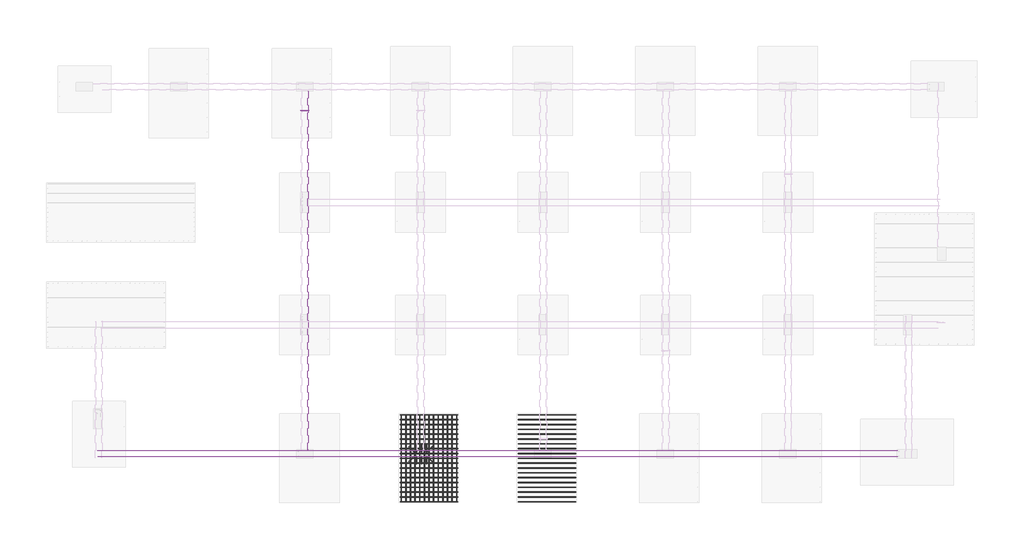
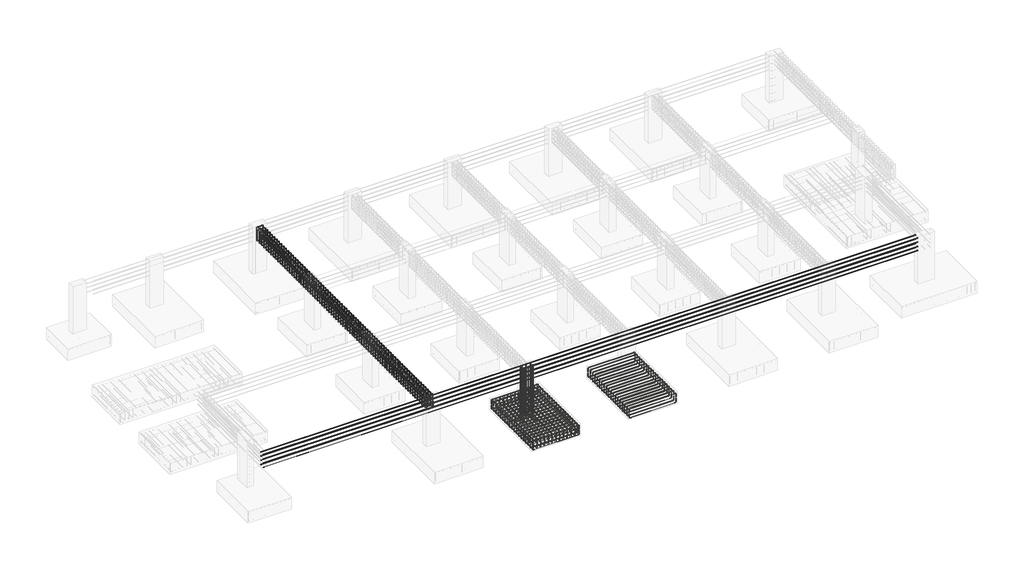
# One storey, part 4 of 16: 16 reinforcing bars.
"""IFC4 building model written with IfcOpenShell, lengths in millimetres."""

from ifc_helpers import new_model, si_unit, point, frame, origin, place, context, project, spatial, polyline, circle_curve, trimmed, segment, composite_curve, source, transform, mapped, element, save
from ifc_brep_helpers import swept_disk

model = new_model("IFC4")

# Units and contexts
model_context = context("Model", 3, world=origin())
ifc_project = project(units=[si_unit("LENGTHUNIT", "METRE", prefix="MILLI")], contexts=[model_context])

# Site, building, storey
site = spatial("IfcSite", under=ifc_project)
building = spatial("IfcBuilding", under=site)
storey = spatial("IfcBuildingStorey", under=building, Elevation=-1828.8)

# Reinforcing bars
placement = place(None, origin())
reinforcing_bar_shape = source(origin(), model_context, "Body", "SolidModel", [
    swept_disk(composite_curve([segment(polyline([(-744.0266166, -5094.4085501, -2088.8), (-744.0266166, -5094.4085501, -2212.8)]), True, "CONTINUOUS"), segment(trimmed(circle_curve(frame((-774.0266166, -5094.4085501, -2212.8), z_axis=(0.0, 1.0, 0.0), x_axis=(30.0, 0.0, 0.0)), 30.0), [point((-744.0266166, -5094.4085501, -2212.8))], [point((-774.0266166, -5094.4085501, -2242.8))], True, "CARTESIAN"), True, "CONTINUOUS"), segment(polyline([(-774.0266166, -5094.4085501, -2242.8), (-2442.0266166, -5094.4085501, -2242.8)]), True, "CONTINUOUS"), segment(trimmed(circle_curve(frame((-2442.0266166, -5094.4085501, -2212.8), z_axis=(0.0, 1.0, 0.0), x_axis=(0.0, 0.0, -30.0)), 30.0), [point((-2442.0266166, -5094.4085501, -2242.8))], [point((-2472.0266166, -5094.4085501, -2212.8))], True, "CARTESIAN"), True, "CONTINUOUS"), segment(polyline([(-2472.0266166, -5094.4085501, -2212.8), (-2472.0266166, -5094.4085501, -2088.8)]), True, "CONTINUOUS")], self_intersect=False), 6.0),
])
element("IfcReinforcingBar", 1, at=placement, inside=storey, context=model_context, shape_type="MappedRepresentation", body=[
    mapped(reinforcing_bar_shape, transform((0.0, 0.0, 0.0), x_axis=(1.0, 0.0, 0.0), y_axis=(0.0, 1.0, 0.0), z_axis=(0.0, 0.0, 1.0))),
    mapped(reinforcing_bar_shape, transform((0.0, -146.0, 0.0), x_axis=(1.0, 0.0, 0.0), y_axis=(0.0, 1.0, 0.0), z_axis=(0.0, 0.0, 1.0))),
    mapped(reinforcing_bar_shape, transform((0.0, -292.0, 0.0), x_axis=(1.0, 0.0, 0.0), y_axis=(0.0, 1.0, 0.0), z_axis=(0.0, 0.0, 1.0))),
    mapped(reinforcing_bar_shape, transform((0.0, -438.0, 0.0), x_axis=(1.0, 0.0, 0.0), y_axis=(0.0, 1.0, 0.0), z_axis=(0.0, 0.0, 1.0))),
    mapped(reinforcing_bar_shape, transform((0.0, -584.0, 0.0), x_axis=(1.0, 0.0, 0.0), y_axis=(0.0, 1.0, 0.0), z_axis=(0.0, 0.0, 1.0))),
    mapped(reinforcing_bar_shape, transform((0.0, -730.0, 0.0), x_axis=(1.0, 0.0, 0.0), y_axis=(0.0, 1.0, 0.0), z_axis=(0.0, 0.0, 1.0))),
    mapped(reinforcing_bar_shape, transform((0.0, -876.0, 0.0), x_axis=(1.0, 0.0, 0.0), y_axis=(0.0, 1.0, 0.0), z_axis=(0.0, 0.0, 1.0))),
    mapped(reinforcing_bar_shape, transform((0.0, -1022.0, 0.0), x_axis=(1.0, 0.0, 0.0), y_axis=(0.0, 1.0, 0.0), z_axis=(0.0, 0.0, 1.0))),
    mapped(reinforcing_bar_shape, transform((0.0, -1168.0, 0.0), x_axis=(1.0, 0.0, 0.0), y_axis=(0.0, 1.0, 0.0), z_axis=(0.0, 0.0, 1.0))),
    mapped(reinforcing_bar_shape, transform((0.0, -1314.0, 0.0), x_axis=(1.0, 0.0, 0.0), y_axis=(0.0, 1.0, 0.0), z_axis=(0.0, 0.0, 1.0))),
    mapped(reinforcing_bar_shape, transform((0.0, -1460.0, 0.0), x_axis=(1.0, 0.0, 0.0), y_axis=(0.0, 1.0, 0.0), z_axis=(0.0, 0.0, 1.0))),
    mapped(reinforcing_bar_shape, transform((0.0, -1606.0, 0.0), x_axis=(1.0, 0.0, 0.0), y_axis=(0.0, 1.0, 0.0), z_axis=(0.0, 0.0, 1.0))),
    mapped(reinforcing_bar_shape, transform((0.0, -1752.0, 0.0), x_axis=(1.0, 0.0, 0.0), y_axis=(0.0, 1.0, 0.0), z_axis=(0.0, 0.0, 1.0))),
    mapped(reinforcing_bar_shape, transform((0.0, -1898.0, 0.0), x_axis=(1.0, 0.0, 0.0), y_axis=(0.0, 1.0, 0.0), z_axis=(0.0, 0.0, 1.0))),
    mapped(reinforcing_bar_shape, transform((0.0, -2044.0, 0.0), x_axis=(1.0, 0.0, 0.0), y_axis=(0.0, 1.0, 0.0), z_axis=(0.0, 0.0, 1.0))),
    mapped(reinforcing_bar_shape, transform((0.0, -2190.0, 0.0), x_axis=(1.0, 0.0, 0.0), y_axis=(0.0, 1.0, 0.0), z_axis=(0.0, 0.0, 1.0))),
    mapped(reinforcing_bar_shape, transform((0.0, -2336.0, 0.0), x_axis=(1.0, 0.0, 0.0), y_axis=(0.0, 1.0, 0.0), z_axis=(0.0, 0.0, 1.0))),
    mapped(reinforcing_bar_shape, transform((0.0, -2482.0, 0.0), x_axis=(1.0, 0.0, 0.0), y_axis=(0.0, 1.0, 0.0), z_axis=(0.0, 0.0, 1.0))),
    mapped(reinforcing_bar_shape, transform((0.0, -2628.0, 0.0), x_axis=(1.0, 0.0, 0.0), y_axis=(0.0, 1.0, 0.0), z_axis=(0.0, 0.0, 1.0))),
])
reinforcing_bar_2_shape = source(origin(), model_context, "Body", "SolidModel", [
    swept_disk(composite_curve([segment(polyline([(-2472.0266166, -5094.4085501, -2024.671783), (-2472.0266166, -5094.4085501, -1900.671783)]), True, "CONTINUOUS"), segment(trimmed(circle_curve(frame((-2442.0266166, -5094.4085501, -1900.671783), z_axis=(0.0, 1.0, 0.0), x_axis=(-30.0, 0.0, 0.0)), 30.0), [point((-2472.0266166, -5094.4085501, -1900.671783))], [point((-2442.0266166, -5094.4085501, -1870.671783))], True, "CARTESIAN"), True, "CONTINUOUS"), segment(polyline([(-2442.0266166, -5094.4085501, -1870.671783), (-774.0266166, -5094.4085501, -1870.671783)]), True, "CONTINUOUS"), segment(trimmed(circle_curve(frame((-774.0266166, -5094.4085501, -1900.671783), z_axis=(0.0, 1.0, 0.0), x_axis=(0.0, 0.0, 30.0)), 30.0), [point((-774.0266166, -5094.4085501, -1870.671783))], [point((-744.0266166, -5094.4085501, -1900.671783))], True, "CARTESIAN"), True, "CONTINUOUS"), segment(polyline([(-744.0266166, -5094.4085501, -1900.671783), (-744.0266166, -5094.4085501, -2024.671783)]), True, "CONTINUOUS")], self_intersect=False), 6.0),
])
element("IfcReinforcingBar", 2, at=placement, inside=storey, context=model_context, shape_type="MappedRepresentation", body=[
    mapped(reinforcing_bar_2_shape, transform((0.0, 0.0, 0.0), x_axis=(1.0, 0.0, 0.0), y_axis=(0.0, 1.0, 0.0), z_axis=(0.0, 0.0, 1.0))),
    mapped(reinforcing_bar_2_shape, transform((0.0, -146.0, 0.0), x_axis=(1.0, 0.0, 0.0), y_axis=(0.0, 1.0, 0.0), z_axis=(0.0, 0.0, 1.0))),
    mapped(reinforcing_bar_2_shape, transform((0.0, -292.0, 0.0), x_axis=(1.0, 0.0, 0.0), y_axis=(0.0, 1.0, 0.0), z_axis=(0.0, 0.0, 1.0))),
    mapped(reinforcing_bar_2_shape, transform((0.0, -438.0, 0.0), x_axis=(1.0, 0.0, 0.0), y_axis=(0.0, 1.0, 0.0), z_axis=(0.0, 0.0, 1.0))),
    mapped(reinforcing_bar_2_shape, transform((0.0, -584.0, 0.0), x_axis=(1.0, 0.0, 0.0), y_axis=(0.0, 1.0, 0.0), z_axis=(0.0, 0.0, 1.0))),
    mapped(reinforcing_bar_2_shape, transform((0.0, -730.0, 0.0), x_axis=(1.0, 0.0, 0.0), y_axis=(0.0, 1.0, 0.0), z_axis=(0.0, 0.0, 1.0))),
    mapped(reinforcing_bar_2_shape, transform((0.0, -876.0, 0.0), x_axis=(1.0, 0.0, 0.0), y_axis=(0.0, 1.0, 0.0), z_axis=(0.0, 0.0, 1.0))),
    mapped(reinforcing_bar_2_shape, transform((0.0, -1022.0, 0.0), x_axis=(1.0, 0.0, 0.0), y_axis=(0.0, 1.0, 0.0), z_axis=(0.0, 0.0, 1.0))),
    mapped(reinforcing_bar_2_shape, transform((0.0, -1168.0, 0.0), x_axis=(1.0, 0.0, 0.0), y_axis=(0.0, 1.0, 0.0), z_axis=(0.0, 0.0, 1.0))),
    mapped(reinforcing_bar_2_shape, transform((0.0, -1314.0, 0.0), x_axis=(1.0, 0.0, 0.0), y_axis=(0.0, 1.0, 0.0), z_axis=(0.0, 0.0, 1.0))),
    mapped(reinforcing_bar_2_shape, transform((0.0, -1460.0, 0.0), x_axis=(1.0, 0.0, 0.0), y_axis=(0.0, 1.0, 0.0), z_axis=(0.0, 0.0, 1.0))),
    mapped(reinforcing_bar_2_shape, transform((0.0, -1606.0, 0.0), x_axis=(1.0, 0.0, 0.0), y_axis=(0.0, 1.0, 0.0), z_axis=(0.0, 0.0, 1.0))),
    mapped(reinforcing_bar_2_shape, transform((0.0, -1752.0, 0.0), x_axis=(1.0, 0.0, 0.0), y_axis=(0.0, 1.0, 0.0), z_axis=(0.0, 0.0, 1.0))),
    mapped(reinforcing_bar_2_shape, transform((0.0, -1898.0, 0.0), x_axis=(1.0, 0.0, 0.0), y_axis=(0.0, 1.0, 0.0), z_axis=(0.0, 0.0, 1.0))),
    mapped(reinforcing_bar_2_shape, transform((0.0, -2044.0, 0.0), x_axis=(1.0, 0.0, 0.0), y_axis=(0.0, 1.0, 0.0), z_axis=(0.0, 0.0, 1.0))),
    mapped(reinforcing_bar_2_shape, transform((0.0, -2190.0, 0.0), x_axis=(1.0, 0.0, 0.0), y_axis=(0.0, 1.0, 0.0), z_axis=(0.0, 0.0, 1.0))),
    mapped(reinforcing_bar_2_shape, transform((0.0, -2336.0, 0.0), x_axis=(1.0, 0.0, 0.0), y_axis=(0.0, 1.0, 0.0), z_axis=(0.0, 0.0, 1.0))),
    mapped(reinforcing_bar_2_shape, transform((0.0, -2482.0, 0.0), x_axis=(1.0, 0.0, 0.0), y_axis=(0.0, 1.0, 0.0), z_axis=(0.0, 0.0, 1.0))),
    mapped(reinforcing_bar_2_shape, transform((0.0, -2628.0, 0.0), x_axis=(1.0, 0.0, 0.0), y_axis=(0.0, 1.0, 0.0), z_axis=(0.0, 0.0, 1.0))),
])
reinforcing_bar_3_shape = source(origin(), model_context, "Body", "SolidModel", [
    swept_disk(composite_curve([segment(polyline([(-4314.2725801, -5094.4085501, -2088.8), (-4314.2725801, -5094.4085501, -2212.8)]), True, "CONTINUOUS"), segment(trimmed(circle_curve(frame((-4344.2725801, -5094.4085501, -2212.8), z_axis=(0.0, 1.0, 0.0), x_axis=(30.0, 0.0, 0.0)), 30.0), [point((-4314.2725801, -5094.4085501, -2212.8))], [point((-4344.2725801, -5094.4085501, -2242.8))], True, "CARTESIAN"), True, "CONTINUOUS"), segment(polyline([(-4344.2725801, -5094.4085501, -2242.8), (-6012.2725801, -5094.4085501, -2242.8)]), True, "CONTINUOUS"), segment(trimmed(circle_curve(frame((-6012.2725801, -5094.4085501, -2212.8), z_axis=(0.0, 1.0, 0.0), x_axis=(0.0, 0.0, -30.0)), 30.0), [point((-6012.2725801, -5094.4085501, -2242.8))], [point((-6042.2725801, -5094.4085501, -2212.8))], True, "CARTESIAN"), True, "CONTINUOUS"), segment(polyline([(-6042.2725801, -5094.4085501, -2212.8), (-6042.2725801, -5094.4085501, -2088.8)]), True, "CONTINUOUS")], self_intersect=False), 6.0),
])
element("IfcReinforcingBar", 3, at=placement, inside=storey, context=model_context, shape_type="MappedRepresentation", body=[
    mapped(reinforcing_bar_3_shape, transform((0.0, 0.0, 0.0), x_axis=(1.0, 0.0, 0.0), y_axis=(0.0, 1.0, 0.0), z_axis=(0.0, 0.0, 1.0))),
    mapped(reinforcing_bar_3_shape, transform((0.0, -146.0, 0.0), x_axis=(1.0, 0.0, 0.0), y_axis=(0.0, 1.0, 0.0), z_axis=(0.0, 0.0, 1.0))),
    mapped(reinforcing_bar_3_shape, transform((0.0, -292.0, 0.0), x_axis=(1.0, 0.0, 0.0), y_axis=(0.0, 1.0, 0.0), z_axis=(0.0, 0.0, 1.0))),
    mapped(reinforcing_bar_3_shape, transform((0.0, -438.0, 0.0), x_axis=(1.0, 0.0, 0.0), y_axis=(0.0, 1.0, 0.0), z_axis=(0.0, 0.0, 1.0))),
    mapped(reinforcing_bar_3_shape, transform((0.0, -584.0, 0.0), x_axis=(1.0, 0.0, 0.0), y_axis=(0.0, 1.0, 0.0), z_axis=(0.0, 0.0, 1.0))),
    mapped(reinforcing_bar_3_shape, transform((0.0, -730.0, 0.0), x_axis=(1.0, 0.0, 0.0), y_axis=(0.0, 1.0, 0.0), z_axis=(0.0, 0.0, 1.0))),
    mapped(reinforcing_bar_3_shape, transform((0.0, -876.0, 0.0), x_axis=(1.0, 0.0, 0.0), y_axis=(0.0, 1.0, 0.0), z_axis=(0.0, 0.0, 1.0))),
    mapped(reinforcing_bar_3_shape, transform((0.0, -1022.0, 0.0), x_axis=(1.0, 0.0, 0.0), y_axis=(0.0, 1.0, 0.0), z_axis=(0.0, 0.0, 1.0))),
    mapped(reinforcing_bar_3_shape, transform((0.0, -1168.0, 0.0), x_axis=(1.0, 0.0, 0.0), y_axis=(0.0, 1.0, 0.0), z_axis=(0.0, 0.0, 1.0))),
    mapped(reinforcing_bar_3_shape, transform((0.0, -1314.0, 0.0), x_axis=(1.0, 0.0, 0.0), y_axis=(0.0, 1.0, 0.0), z_axis=(0.0, 0.0, 1.0))),
    mapped(reinforcing_bar_3_shape, transform((0.0, -1460.0, 0.0), x_axis=(1.0, 0.0, 0.0), y_axis=(0.0, 1.0, 0.0), z_axis=(0.0, 0.0, 1.0))),
    mapped(reinforcing_bar_3_shape, transform((0.0, -1606.0, 0.0), x_axis=(1.0, 0.0, 0.0), y_axis=(0.0, 1.0, 0.0), z_axis=(0.0, 0.0, 1.0))),
    mapped(reinforcing_bar_3_shape, transform((0.0, -1752.0, 0.0), x_axis=(1.0, 0.0, 0.0), y_axis=(0.0, 1.0, 0.0), z_axis=(0.0, 0.0, 1.0))),
    mapped(reinforcing_bar_3_shape, transform((0.0, -1898.0, 0.0), x_axis=(1.0, 0.0, 0.0), y_axis=(0.0, 1.0, 0.0), z_axis=(0.0, 0.0, 1.0))),
    mapped(reinforcing_bar_3_shape, transform((0.0, -2044.0, 0.0), x_axis=(1.0, 0.0, 0.0), y_axis=(0.0, 1.0, 0.0), z_axis=(0.0, 0.0, 1.0))),
    mapped(reinforcing_bar_3_shape, transform((0.0, -2190.0, 0.0), x_axis=(1.0, 0.0, 0.0), y_axis=(0.0, 1.0, 0.0), z_axis=(0.0, 0.0, 1.0))),
    mapped(reinforcing_bar_3_shape, transform((0.0, -2336.0, 0.0), x_axis=(1.0, 0.0, 0.0), y_axis=(0.0, 1.0, 0.0), z_axis=(0.0, 0.0, 1.0))),
    mapped(reinforcing_bar_3_shape, transform((0.0, -2482.0, 0.0), x_axis=(1.0, 0.0, 0.0), y_axis=(0.0, 1.0, 0.0), z_axis=(0.0, 0.0, 1.0))),
    mapped(reinforcing_bar_3_shape, transform((0.0, -2628.0, 0.0), x_axis=(1.0, 0.0, 0.0), y_axis=(0.0, 1.0, 0.0), z_axis=(0.0, 0.0, 1.0))),
])
reinforcing_bar_4_shape = source(origin(), model_context, "Body", "SolidModel", [
    swept_disk(composite_curve([segment(polyline([(-6042.2725801, -5094.4085501, -2024.671783), (-6042.2725801, -5094.4085501, -1900.671783)]), True, "CONTINUOUS"), segment(trimmed(circle_curve(frame((-6012.2725801, -5094.4085501, -1900.671783), z_axis=(0.0, 1.0, 0.0), x_axis=(-30.0, 0.0, 0.0)), 30.0), [point((-6042.2725801, -5094.4085501, -1900.671783))], [point((-6012.2725801, -5094.4085501, -1870.671783))], True, "CARTESIAN"), True, "CONTINUOUS"), segment(polyline([(-6012.2725801, -5094.4085501, -1870.671783), (-4344.2725801, -5094.4085501, -1870.671783)]), True, "CONTINUOUS"), segment(trimmed(circle_curve(frame((-4344.2725801, -5094.4085501, -1900.671783), z_axis=(0.0, 1.0, 0.0), x_axis=(0.0, 0.0, 30.0)), 30.0), [point((-4344.2725801, -5094.4085501, -1870.671783))], [point((-4314.2725801, -5094.4085501, -1900.671783))], True, "CARTESIAN"), True, "CONTINUOUS"), segment(polyline([(-4314.2725801, -5094.4085501, -1900.671783), (-4314.2725801, -5094.4085501, -2024.671783)]), True, "CONTINUOUS")], self_intersect=False), 6.0),
])
element("IfcReinforcingBar", 4, at=placement, inside=storey, context=model_context, shape_type="MappedRepresentation", body=[
    mapped(reinforcing_bar_4_shape, transform((0.0, 0.0, 0.0), x_axis=(1.0, 0.0, 0.0), y_axis=(0.0, 1.0, 0.0), z_axis=(0.0, 0.0, 1.0))),
    mapped(reinforcing_bar_4_shape, transform((0.0, -146.0, 0.0), x_axis=(1.0, 0.0, 0.0), y_axis=(0.0, 1.0, 0.0), z_axis=(0.0, 0.0, 1.0))),
    mapped(reinforcing_bar_4_shape, transform((0.0, -292.0, 0.0), x_axis=(1.0, 0.0, 0.0), y_axis=(0.0, 1.0, 0.0), z_axis=(0.0, 0.0, 1.0))),
    mapped(reinforcing_bar_4_shape, transform((0.0, -438.0, 0.0), x_axis=(1.0, 0.0, 0.0), y_axis=(0.0, 1.0, 0.0), z_axis=(0.0, 0.0, 1.0))),
    mapped(reinforcing_bar_4_shape, transform((0.0, -584.0, 0.0), x_axis=(1.0, 0.0, 0.0), y_axis=(0.0, 1.0, 0.0), z_axis=(0.0, 0.0, 1.0))),
    mapped(reinforcing_bar_4_shape, transform((0.0, -730.0, 0.0), x_axis=(1.0, 0.0, 0.0), y_axis=(0.0, 1.0, 0.0), z_axis=(0.0, 0.0, 1.0))),
    mapped(reinforcing_bar_4_shape, transform((0.0, -876.0, 0.0), x_axis=(1.0, 0.0, 0.0), y_axis=(0.0, 1.0, 0.0), z_axis=(0.0, 0.0, 1.0))),
    mapped(reinforcing_bar_4_shape, transform((0.0, -1022.0, 0.0), x_axis=(1.0, 0.0, 0.0), y_axis=(0.0, 1.0, 0.0), z_axis=(0.0, 0.0, 1.0))),
    mapped(reinforcing_bar_4_shape, transform((0.0, -1168.0, 0.0), x_axis=(1.0, 0.0, 0.0), y_axis=(0.0, 1.0, 0.0), z_axis=(0.0, 0.0, 1.0))),
    mapped(reinforcing_bar_4_shape, transform((0.0, -1314.0, 0.0), x_axis=(1.0, 0.0, 0.0), y_axis=(0.0, 1.0, 0.0), z_axis=(0.0, 0.0, 1.0))),
    mapped(reinforcing_bar_4_shape, transform((0.0, -1460.0, 0.0), x_axis=(1.0, 0.0, 0.0), y_axis=(0.0, 1.0, 0.0), z_axis=(0.0, 0.0, 1.0))),
    mapped(reinforcing_bar_4_shape, transform((0.0, -1606.0, 0.0), x_axis=(1.0, 0.0, 0.0), y_axis=(0.0, 1.0, 0.0), z_axis=(0.0, 0.0, 1.0))),
    mapped(reinforcing_bar_4_shape, transform((0.0, -1752.0, 0.0), x_axis=(1.0, 0.0, 0.0), y_axis=(0.0, 1.0, 0.0), z_axis=(0.0, 0.0, 1.0))),
    mapped(reinforcing_bar_4_shape, transform((0.0, -1898.0, 0.0), x_axis=(1.0, 0.0, 0.0), y_axis=(0.0, 1.0, 0.0), z_axis=(0.0, 0.0, 1.0))),
    mapped(reinforcing_bar_4_shape, transform((0.0, -2044.0, 0.0), x_axis=(1.0, 0.0, 0.0), y_axis=(0.0, 1.0, 0.0), z_axis=(0.0, 0.0, 1.0))),
    mapped(reinforcing_bar_4_shape, transform((0.0, -2190.0, 0.0), x_axis=(1.0, 0.0, 0.0), y_axis=(0.0, 1.0, 0.0), z_axis=(0.0, 0.0, 1.0))),
    mapped(reinforcing_bar_4_shape, transform((0.0, -2336.0, 0.0), x_axis=(1.0, 0.0, 0.0), y_axis=(0.0, 1.0, 0.0), z_axis=(0.0, 0.0, 1.0))),
    mapped(reinforcing_bar_4_shape, transform((0.0, -2482.0, 0.0), x_axis=(1.0, 0.0, 0.0), y_axis=(0.0, 1.0, 0.0), z_axis=(0.0, 0.0, 1.0))),
    mapped(reinforcing_bar_4_shape, transform((0.0, -2628.0, 0.0), x_axis=(1.0, 0.0, 0.0), y_axis=(0.0, 1.0, 0.0), z_axis=(0.0, 0.0, 1.0))),
])
reinforcing_bar_5_shape = source(origin(), model_context, "Body", "SolidModel", [
    swept_disk(composite_curve([segment(polyline([(-6015.8984804, -5094.4085501, -2074.8303715), (-6015.8984804, -5094.4085501, -2198.8303715)]), True, "CONTINUOUS"), segment(trimmed(circle_curve(frame((-6015.8984804, -5124.4085501, -2198.8303715), z_axis=(-1.0, 0.0, 0.0), x_axis=(0.0, 30.0, 0.0)), 30.0), [point((-6015.8984804, -5094.4085501, -2198.8303715))], [point((-6015.8984804, -5124.4085501, -2228.8303715))], True, "CARTESIAN"), True, "CONTINUOUS"), segment(polyline([(-6015.8984804, -5124.4085501, -2228.8303715), (-6015.8984804, -7692.4085501, -2228.8303715)]), True, "CONTINUOUS"), segment(trimmed(circle_curve(frame((-6015.8984804, -7692.4085501, -2198.8303715), z_axis=(-1.0, 0.0, 0.0), x_axis=(0.0, 0.0, -30.0)), 30.0), [point((-6015.8984804, -7692.4085501, -2228.8303715))], [point((-6015.8984804, -7722.4085501, -2198.8303715))], True, "CARTESIAN"), True, "CONTINUOUS"), segment(polyline([(-6015.8984804, -7722.4085501, -2198.8303715), (-6015.8984804, -7722.4085501, -2074.8303715)]), True, "CONTINUOUS")], self_intersect=False), 6.0),
])
element("IfcReinforcingBar", 5, at=placement, inside=storey, context=model_context, shape_type="MappedRepresentation", body=[
    mapped(reinforcing_bar_5_shape, transform((0.0, 0.0, 0.0), x_axis=(1.0, 0.0, 0.0), y_axis=(0.0, 1.0, 0.0), z_axis=(0.0, 0.0, 1.0))),
    mapped(reinforcing_bar_5_shape, transform((139.7704391, 0.0, 0.0), x_axis=(1.0, 0.0, 0.0), y_axis=(0.0, 1.0, 0.0), z_axis=(0.0, 0.0, 1.0))),
    mapped(reinforcing_bar_5_shape, transform((279.5408781, 0.0, 0.0), x_axis=(1.0, 0.0, 0.0), y_axis=(0.0, 1.0, 0.0), z_axis=(0.0, 0.0, 1.0))),
    mapped(reinforcing_bar_5_shape, transform((419.3113172, 0.0, 0.0), x_axis=(1.0, 0.0, 0.0), y_axis=(0.0, 1.0, 0.0), z_axis=(0.0, 0.0, 1.0))),
    mapped(reinforcing_bar_5_shape, transform((559.0817562, 0.0, 0.0), x_axis=(1.0, 0.0, 0.0), y_axis=(0.0, 1.0, 0.0), z_axis=(0.0, 0.0, 1.0))),
    mapped(reinforcing_bar_5_shape, transform((698.8521953, 0.0, 0.0), x_axis=(1.0, 0.0, 0.0), y_axis=(0.0, 1.0, 0.0), z_axis=(0.0, 0.0, 1.0))),
    mapped(reinforcing_bar_5_shape, transform((838.6226343, 0.0, 0.0), x_axis=(1.0, 0.0, 0.0), y_axis=(0.0, 1.0, 0.0), z_axis=(0.0, 0.0, 1.0))),
    mapped(reinforcing_bar_5_shape, transform((978.3930734, 0.0, 0.0), x_axis=(1.0, 0.0, 0.0), y_axis=(0.0, 1.0, 0.0), z_axis=(0.0, 0.0, 1.0))),
    mapped(reinforcing_bar_5_shape, transform((1118.1635125, 0.0, 0.0), x_axis=(1.0, 0.0, 0.0), y_axis=(0.0, 1.0, 0.0), z_axis=(0.0, 0.0, 1.0))),
    mapped(reinforcing_bar_5_shape, transform((1257.9339515, 0.0, 0.0), x_axis=(1.0, 0.0, 0.0), y_axis=(0.0, 1.0, 0.0), z_axis=(0.0, 0.0, 1.0))),
    mapped(reinforcing_bar_5_shape, transform((1397.7043906, 0.0, 0.0), x_axis=(1.0, 0.0, 0.0), y_axis=(0.0, 1.0, 0.0), z_axis=(0.0, 0.0, 1.0))),
    mapped(reinforcing_bar_5_shape, transform((1537.4748296, 0.0, 0.0), x_axis=(1.0, 0.0, 0.0), y_axis=(0.0, 1.0, 0.0), z_axis=(0.0, 0.0, 1.0))),
    mapped(reinforcing_bar_5_shape, transform((1677.2452687, 0.0, 0.0), x_axis=(1.0, 0.0, 0.0), y_axis=(0.0, 1.0, 0.0), z_axis=(0.0, 0.0, 1.0))),
])
reinforcing_bar_6_shape = source(origin(), model_context, "Body", "SolidModel", [
    swept_disk(composite_curve([segment(polyline([(-4338.6532117, -5094.4085501, -2038.9453456), (-4338.6532117, -5094.4085501, -1914.9453456)]), True, "CONTINUOUS"), segment(trimmed(circle_curve(frame((-4338.6532117, -5124.4085501, -1914.9453456), z_axis=(1.0, 0.0, 0.0), x_axis=(0.0, 30.0, 0.0)), 30.0), [point((-4338.6532117, -5094.4085501, -1914.9453456))], [point((-4338.6532117, -5124.4085501, -1884.9453456))], True, "CARTESIAN"), True, "CONTINUOUS"), segment(polyline([(-4338.6532117, -5124.4085501, -1884.9453456), (-4338.6532117, -7692.4085501, -1884.9453456)]), True, "CONTINUOUS"), segment(trimmed(circle_curve(frame((-4338.6532117, -7692.4085501, -1914.9453456), z_axis=(1.0, 0.0, 0.0), x_axis=(0.0, 0.0, 30.0)), 30.0), [point((-4338.6532117, -7692.4085501, -1884.9453456))], [point((-4338.6532117, -7722.4085501, -1914.9453456))], True, "CARTESIAN"), True, "CONTINUOUS"), segment(polyline([(-4338.6532117, -7722.4085501, -1914.9453456), (-4338.6532117, -7722.4085501, -2038.9453456)]), True, "CONTINUOUS")], self_intersect=False), 6.0),
])
element("IfcReinforcingBar", 6, at=placement, inside=storey, context=model_context, shape_type="MappedRepresentation", body=[
    mapped(reinforcing_bar_6_shape, transform((0.0, 0.0, 0.0), x_axis=(1.0, 0.0, 0.0), y_axis=(0.0, 1.0, 0.0), z_axis=(0.0, 0.0, 1.0))),
    mapped(reinforcing_bar_6_shape, transform((-139.7704391, 0.0, 0.0), x_axis=(1.0, 0.0, 0.0), y_axis=(0.0, 1.0, 0.0), z_axis=(0.0, 0.0, 1.0))),
    mapped(reinforcing_bar_6_shape, transform((-279.5408781, 0.0, 0.0), x_axis=(1.0, 0.0, 0.0), y_axis=(0.0, 1.0, 0.0), z_axis=(0.0, 0.0, 1.0))),
    mapped(reinforcing_bar_6_shape, transform((-419.3113172, 0.0, 0.0), x_axis=(1.0, 0.0, 0.0), y_axis=(0.0, 1.0, 0.0), z_axis=(0.0, 0.0, 1.0))),
    mapped(reinforcing_bar_6_shape, transform((-559.0817562, 0.0, 0.0), x_axis=(1.0, 0.0, 0.0), y_axis=(0.0, 1.0, 0.0), z_axis=(0.0, 0.0, 1.0))),
    mapped(reinforcing_bar_6_shape, transform((-698.8521953, 0.0, 0.0), x_axis=(1.0, 0.0, 0.0), y_axis=(0.0, 1.0, 0.0), z_axis=(0.0, 0.0, 1.0))),
    mapped(reinforcing_bar_6_shape, transform((-838.6226343, 0.0, 0.0), x_axis=(1.0, 0.0, 0.0), y_axis=(0.0, 1.0, 0.0), z_axis=(0.0, 0.0, 1.0))),
    mapped(reinforcing_bar_6_shape, transform((-978.3930734, 0.0, 0.0), x_axis=(1.0, 0.0, 0.0), y_axis=(0.0, 1.0, 0.0), z_axis=(0.0, 0.0, 1.0))),
    mapped(reinforcing_bar_6_shape, transform((-1118.1635125, 0.0, 0.0), x_axis=(1.0, 0.0, 0.0), y_axis=(0.0, 1.0, 0.0), z_axis=(0.0, 0.0, 1.0))),
    mapped(reinforcing_bar_6_shape, transform((-1257.9339515, 0.0, 0.0), x_axis=(1.0, 0.0, 0.0), y_axis=(0.0, 1.0, 0.0), z_axis=(0.0, 0.0, 1.0))),
    mapped(reinforcing_bar_6_shape, transform((-1397.7043906, 0.0, 0.0), x_axis=(1.0, 0.0, 0.0), y_axis=(0.0, 1.0, 0.0), z_axis=(0.0, 0.0, 1.0))),
    mapped(reinforcing_bar_6_shape, transform((-1537.4748296, 0.0, 0.0), x_axis=(1.0, 0.0, 0.0), y_axis=(0.0, 1.0, 0.0), z_axis=(0.0, 0.0, 1.0))),
    mapped(reinforcing_bar_6_shape, transform((-1677.2452687, 0.0, 0.0), x_axis=(1.0, 0.0, 0.0), y_axis=(0.0, 1.0, 0.0), z_axis=(0.0, 0.0, 1.0))),
])
reinforcing_bar_7_shape = source(origin(), model_context, "Body", "SolidModel", [
    swept_disk(composite_curve([segment(polyline([(-5560.102427, -6208.8808991, -30.0), (-5560.102427, -6208.8808991, -2141.7459972)]), True, "CONTINUOUS"), segment(trimmed(circle_curve(frame((-5560.102427, -6178.8808991, -2141.7459972), z_axis=(1.0, 0.0, 0.0), x_axis=(0.0, -30.0, 0.0)), 30.0), [point((-5560.102427, -6208.8808991, -2141.7459972))], [point((-5560.102427, -6178.8808991, -2171.7459972))], True, "CARTESIAN"), True, "CONTINUOUS"), segment(polyline([(-5560.102427, -6178.8808991, -2171.7459972), (-5560.102427, -5988.2528007, -2171.7459972)]), True, "CONTINUOUS")], self_intersect=False), 6.0),
])
element("IfcReinforcingBar", 7, at=placement, inside=storey, context=model_context, shape_type="MappedRepresentation", body=[
    mapped(reinforcing_bar_7_shape, transform((0.0, 0.0, 0.0), x_axis=(1.0, 0.0, 0.0), y_axis=(0.0, 1.0, 0.0), z_axis=(0.0, 0.0, 1.0))),
    mapped(reinforcing_bar_7_shape, transform((153.9273626, 0.0, 0.0), x_axis=(1.0, 0.0, 0.0), y_axis=(0.0, 1.0, 0.0), z_axis=(0.0, 0.0, 1.0))),
    mapped(reinforcing_bar_7_shape, transform((307.8547253, 0.0, 0.0), x_axis=(1.0, 0.0, 0.0), y_axis=(0.0, 1.0, 0.0), z_axis=(0.0, 0.0, 1.0))),
])
element("IfcReinforcingBar", 8, at=placement, inside=storey, context=model_context, shape_type="SolidModel", body=[
    swept_disk(composite_curve([segment(polyline([(-5621.7720578, -6208.8808991, -30.0), (-5621.7720578, -6208.8808991, -2141.7459972)]), True, "CONTINUOUS"), segment(trimmed(circle_curve(frame((-5642.9852612, -6187.6676957, -2141.7459972), z_axis=(0.7071067811865477, 0.7071067811865474, 0.0), x_axis=(21.213203400000566, -21.213203399999657, 0.0)), 30.0), [point((-5621.7720578, -6208.8808991, -2141.7459972))], [point((-5642.9852612, -6187.6676957, -2171.7459972))], True, "CARTESIAN"), True, "CONTINUOUS"), segment(polyline([(-5642.9852612, -6187.6676957, -2171.7459972), (-5777.7796823, -6052.8732746, -2171.7459972)]), True, "CONTINUOUS")], self_intersect=False), 6.0),
])
element("IfcReinforcingBar", 9, at=placement, inside=storey, context=model_context, shape_type="SolidModel", body=[
    swept_disk(composite_curve([segment(polyline([(-5621.7720578, -6349.3808991, -30.0), (-5621.7720578, -6349.3808991, -2141.7459972)]), True, "CONTINUOUS"), segment(trimmed(circle_curve(frame((-5642.9852612, -6370.5941026, -2141.7459972), z_axis=(-0.7071067811865445, 0.7071067811865507, 0.0), x_axis=(21.213203400000566, 21.213203500000418, 0.0)), 30.0), [point((-5621.7720578, -6349.3808991, -2141.7459972))], [point((-5642.9852612, -6370.5941026, -2171.7459972))], True, "CARTESIAN"), True, "CONTINUOUS"), segment(polyline([(-5642.9852612, -6370.5941026, -2171.7459972), (-5777.7796823, -6505.3885237, -2171.7459972)]), True, "CONTINUOUS")], self_intersect=False), 6.0),
])
element("IfcReinforcingBar", 10, at=placement, inside=storey, context=model_context, shape_type="SolidModel", body=[
    swept_disk(composite_curve([segment(polyline([(-5234.7731024, -6349.3808991, -30.0), (-5234.7731024, -6349.3808991, -2141.7459972)]), True, "CONTINUOUS"), segment(trimmed(circle_curve(frame((-5213.559899, -6370.5941026, -2141.7459972), z_axis=(-0.7071067811865445, -0.7071067811865506, 0.0), x_axis=(-21.213203400000566, 21.213203500000418, 0.0)), 30.0), [point((-5234.7731024, -6349.3808991, -2141.7459972))], [point((-5213.559899, -6370.5941026, -2171.7459972))], True, "CARTESIAN"), True, "CONTINUOUS"), segment(polyline([(-5213.559899, -6370.5941026, -2171.7459972), (-5078.7654779, -6505.3885237, -2171.7459972)]), True, "CONTINUOUS")], self_intersect=False), 6.0),
])
element("IfcReinforcingBar", 11, at=placement, inside=storey, context=model_context, shape_type="SolidModel", body=[
    swept_disk(composite_curve([segment(polyline([(-5234.7731024, -6208.8808991, -30.0), (-5234.7731024, -6208.8808991, -2141.7459972)]), True, "CONTINUOUS"), segment(trimmed(circle_curve(frame((-5213.559899, -6187.6676957, -2141.7459972), z_axis=(0.7071067811865476, -0.7071067811865475, 0.0), x_axis=(-21.213203400000566, -21.213203399999657, 0.0)), 30.0), [point((-5234.7731024, -6208.8808991, -2141.7459972))], [point((-5213.559899, -6187.6676957, -2171.7459972))], True, "CARTESIAN"), True, "CONTINUOUS"), segment(polyline([(-5213.559899, -6187.6676957, -2171.7459972), (-5078.7654779, -6052.8732746, -2171.7459972)]), True, "CONTINUOUS")], self_intersect=False), 6.0),
])
reinforcing_bar_8_shape = source(origin(), model_context, "Body", "SolidModel", [
    swept_disk(composite_curve([segment(polyline([(-5560.102427, -6349.3808991, -30.0), (-5560.102427, -6349.3808991, -2141.7459972)]), True, "CONTINUOUS"), segment(trimmed(circle_curve(frame((-5560.102427, -6379.3808991, -2141.7459972), z_axis=(-1.0, 0.0, 0.0), x_axis=(0.0, 30.0, 0.0)), 30.0), [point((-5560.102427, -6349.3808991, -2141.7459972))], [point((-5560.102427, -6379.3808991, -2171.7459972))], True, "CARTESIAN"), True, "CONTINUOUS"), segment(polyline([(-5560.102427, -6379.3808991, -2171.7459972), (-5560.102427, -6570.0089976, -2171.7459972)]), True, "CONTINUOUS")], self_intersect=False), 6.0),
])
element("IfcReinforcingBar", 12, at=placement, inside=storey, context=model_context, shape_type="MappedRepresentation", body=[
    mapped(reinforcing_bar_8_shape, transform((0.0, 0.0, 0.0), x_axis=(1.0, 0.0, 0.0), y_axis=(0.0, 1.0, 0.0), z_axis=(0.0, 0.0, 1.0))),
    mapped(reinforcing_bar_8_shape, transform((153.9273626, 0.0, 0.0), x_axis=(1.0, 0.0, 0.0), y_axis=(0.0, 1.0, 0.0), z_axis=(0.0, 0.0, 1.0))),
    mapped(reinforcing_bar_8_shape, transform((307.8547253, 0.0, 0.0), x_axis=(1.0, 0.0, 0.0), y_axis=(0.0, 1.0, 0.0), z_axis=(0.0, 0.0, 1.0))),
])
reinforcing_bar_9_shape = source(origin(), model_context, "Body", "SolidModel", [
    swept_disk(composite_curve([segment(polyline([(8986.6771863, -6176.2514249, -53.2720779), (-15177.4472168, -6176.2514249, -53.2720779)]), True, "CONTINUOUS")], self_intersect=False), 6.0),
])
element("IfcReinforcingBar", 13, at=placement, inside=storey, context=model_context, shape_type="MappedRepresentation", body=[
    mapped(reinforcing_bar_9_shape, transform((0.0, 0.0, 0.0), x_axis=(1.0, 0.0, 0.0), y_axis=(0.0, 1.0, 0.0), z_axis=(0.0, 0.0, 1.0))),
    mapped(reinforcing_bar_9_shape, transform((0.0, 0.0, -164.4852814), x_axis=(1.0, 0.0, 0.0), y_axis=(0.0, 1.0, 0.0), z_axis=(0.0, 0.0, 1.0))),
    mapped(reinforcing_bar_9_shape, transform((0.0, 0.0, -328.9705627), x_axis=(1.0, 0.0, 0.0), y_axis=(0.0, 1.0, 0.0), z_axis=(0.0, 0.0, 1.0))),
    mapped(reinforcing_bar_9_shape, transform((0.0, 0.0, -493.4558441), x_axis=(1.0, 0.0, 0.0), y_axis=(0.0, 1.0, 0.0), z_axis=(0.0, 0.0, 1.0))),
])
reinforcing_bar_10_shape = source(origin(), model_context, "Body", "SolidModel", [
    swept_disk(composite_curve([segment(polyline([(8964.5472196, -6350.8588212, -546.7279221), (-15186.9488898, -6350.8588212, -546.7279221)]), True, "CONTINUOUS")], self_intersect=False), 6.0),
])
element("IfcReinforcingBar", 14, at=placement, inside=storey, context=model_context, shape_type="MappedRepresentation", body=[
    mapped(reinforcing_bar_10_shape, transform((0.0, 0.0, 0.0), x_axis=(1.0, 0.0, 0.0), y_axis=(0.0, 1.0, 0.0), z_axis=(0.0, 0.0, 1.0))),
    mapped(reinforcing_bar_10_shape, transform((0.0, 0.0, 164.4852814), x_axis=(1.0, 0.0, 0.0), y_axis=(0.0, 1.0, 0.0), z_axis=(0.0, 0.0, 1.0))),
    mapped(reinforcing_bar_10_shape, transform((0.0, 0.0, 328.9705627), x_axis=(1.0, 0.0, 0.0), y_axis=(0.0, 1.0, 0.0), z_axis=(0.0, 0.0, 1.0))),
    mapped(reinforcing_bar_10_shape, transform((0.0, 0.0, 493.4558441), x_axis=(1.0, 0.0, 0.0), y_axis=(0.0, 1.0, 0.0), z_axis=(0.0, 0.0, 1.0))),
])
reinforcing_bar_11_shape = source(origin(), model_context, "Body", "SolidModel", [
    swept_disk(composite_curve([segment(polyline([(-8903.3781358, 4695.8691009, -132.4680374), (-8991.0593767, 4695.8691009, -44.7867966)]), True, "CONTINUOUS"), segment(trimmed(circle_curve(frame((-9012.2725801, 4695.8691009, -66.0), z_axis=(0.0, -1.0, 0.0), x_axis=(21.213203400000566, 0.0, 21.213203399999998)), 30.0), [point((-8991.0593767, 4695.8691009, -44.7867966))], [point((-9042.2725801, 4695.8691009, -66.0))], True, "CARTESIAN"), True, "CONTINUOUS"), segment(polyline([(-9042.2725801, 4695.8691009, -66.0), (-9042.2725801, 4695.8691009, -534.0)]), True, "CONTINUOUS"), segment(trimmed(circle_curve(frame((-9012.2725801, 4695.8691009, -534.0), z_axis=(0.0, -1.0, 0.0), x_axis=(-30.0, 0.0, 0.0)), 30.0), [point((-9042.2725801, 4695.8691009, -534.0))], [point((-9012.2725801, 4695.8691009, -564.0))], True, "CARTESIAN"), True, "CONTINUOUS"), segment(polyline([(-9012.2725801, 4695.8691009, -564.0), (-8844.2725801, 4695.8691009, -564.0)]), True, "CONTINUOUS"), segment(trimmed(circle_curve(frame((-8844.2725801, 4696.550743, -534.0077449), z_axis=(0.0, -0.9997418355449428, 0.022721405353294154), x_axis=(0.0, -0.681642099999408, -29.992255099999966)), 30.0), [point((-8844.2725801, 4695.8691009, -564.0))], [point((-8814.2725801, 4696.550743, -534.0077449))], True, "CARTESIAN"), True, "CONTINUOUS"), segment(polyline([(-8814.2725801, 4696.550743, -534.0077449), (-8814.2725801, 4707.1874587, -65.9922551)]), True, "CONTINUOUS"), segment(trimmed(circle_curve(frame((-8844.2725801, 4707.1874587, -65.9922551), z_axis=(0.0, -0.9997418355449428, 0.022721405353294154), x_axis=(30.0, 0.0, 0.0)), 30.0), [point((-8814.2725801, 4707.1874587, -65.9922551))], [point((-8844.2725801, 4707.8691009, -36.0))], True, "CARTESIAN"), True, "CONTINUOUS"), segment(polyline([(-8844.2725801, 4707.8691009, -36.0), (-9012.2725801, 4707.8691009, -36.0)]), True, "CONTINUOUS"), segment(trimmed(circle_curve(frame((-9012.2725801, 4707.8691009, -66.0), z_axis=(0.0, -1.0, 0.0), x_axis=(0.0, 0.0, 30.0)), 30.0), [point((-9012.2725801, 4707.8691009, -36.0))], [point((-9033.4857835, 4707.8691009, -87.2132034))], True, "CARTESIAN"), True, "CONTINUOUS"), segment(polyline([(-9033.4857835, 4707.8691009, -87.2132034), (-8945.8045427, 4707.8691009, -174.8944443)]), True, "CONTINUOUS")], self_intersect=False), 6.0),
])
element("IfcReinforcingBar", 15, at=placement, inside=storey, context=model_context, shape_type="MappedRepresentation", body=[
    mapped(reinforcing_bar_11_shape, transform((0.0, 0.0, 0.0), x_axis=(1.0, 0.0, 0.0), y_axis=(0.0, 1.0, 0.0), z_axis=(0.0, 0.0, 1.0))),
    mapped(reinforcing_bar_11_shape, transform((0.0, -148.630137, 0.0), x_axis=(1.0, 0.0, 0.0), y_axis=(0.0, 1.0, 0.0), z_axis=(0.0, 0.0, 1.0))),
    mapped(reinforcing_bar_11_shape, transform((0.0, -297.260274, 0.0), x_axis=(1.0, 0.0, 0.0), y_axis=(0.0, 1.0, 0.0), z_axis=(0.0, 0.0, 1.0))),
    mapped(reinforcing_bar_11_shape, transform((0.0, -445.890411, 0.0), x_axis=(1.0, 0.0, 0.0), y_axis=(0.0, 1.0, 0.0), z_axis=(0.0, 0.0, 1.0))),
    mapped(reinforcing_bar_11_shape, transform((0.0, -594.5205479, 0.0), x_axis=(1.0, 0.0, 0.0), y_axis=(0.0, 1.0, 0.0), z_axis=(0.0, 0.0, 1.0))),
    mapped(reinforcing_bar_11_shape, transform((0.0, -743.1506849, 0.0), x_axis=(1.0, 0.0, 0.0), y_axis=(0.0, 1.0, 0.0), z_axis=(0.0, 0.0, 1.0))),
    mapped(reinforcing_bar_11_shape, transform((0.0, -891.7808219, 0.0), x_axis=(1.0, 0.0, 0.0), y_axis=(0.0, 1.0, 0.0), z_axis=(0.0, 0.0, 1.0))),
    mapped(reinforcing_bar_11_shape, transform((0.0, -1040.4109589, 0.0), x_axis=(1.0, 0.0, 0.0), y_axis=(0.0, 1.0, 0.0), z_axis=(0.0, 0.0, 1.0))),
    mapped(reinforcing_bar_11_shape, transform((0.0, -1189.0410959, 0.0), x_axis=(1.0, 0.0, 0.0), y_axis=(0.0, 1.0, 0.0), z_axis=(0.0, 0.0, 1.0))),
    mapped(reinforcing_bar_11_shape, transform((0.0, -1337.6712329, 0.0), x_axis=(1.0, 0.0, 0.0), y_axis=(0.0, 1.0, 0.0), z_axis=(0.0, 0.0, 1.0))),
    mapped(reinforcing_bar_11_shape, transform((0.0, -1486.3013699, 0.0), x_axis=(1.0, 0.0, 0.0), y_axis=(0.0, 1.0, 0.0), z_axis=(0.0, 0.0, 1.0))),
    mapped(reinforcing_bar_11_shape, transform((0.0, -1634.9315069, 0.0), x_axis=(1.0, 0.0, 0.0), y_axis=(0.0, 1.0, 0.0), z_axis=(0.0, 0.0, 1.0))),
    mapped(reinforcing_bar_11_shape, transform((0.0, -1783.5616438, 0.0), x_axis=(1.0, 0.0, 0.0), y_axis=(0.0, 1.0, 0.0), z_axis=(0.0, 0.0, 1.0))),
    mapped(reinforcing_bar_11_shape, transform((0.0, -1932.1917808, 0.0), x_axis=(1.0, 0.0, 0.0), y_axis=(0.0, 1.0, 0.0), z_axis=(0.0, 0.0, 1.0))),
    mapped(reinforcing_bar_11_shape, transform((0.0, -2080.8219178, 0.0), x_axis=(1.0, 0.0, 0.0), y_axis=(0.0, 1.0, 0.0), z_axis=(0.0, 0.0, 1.0))),
    mapped(reinforcing_bar_11_shape, transform((0.0, -2229.4520548, 0.0), x_axis=(1.0, 0.0, 0.0), y_axis=(0.0, 1.0, 0.0), z_axis=(0.0, 0.0, 1.0))),
    mapped(reinforcing_bar_11_shape, transform((0.0, -2378.0821918, 0.0), x_axis=(1.0, 0.0, 0.0), y_axis=(0.0, 1.0, 0.0), z_axis=(0.0, 0.0, 1.0))),
    mapped(reinforcing_bar_11_shape, transform((0.0, -2526.7123288, 0.0), x_axis=(1.0, 0.0, 0.0), y_axis=(0.0, 1.0, 0.0), z_axis=(0.0, 0.0, 1.0))),
    mapped(reinforcing_bar_11_shape, transform((0.0, -2675.3424658, 0.0), x_axis=(1.0, 0.0, 0.0), y_axis=(0.0, 1.0, 0.0), z_axis=(0.0, 0.0, 1.0))),
    mapped(reinforcing_bar_11_shape, transform((0.0, -2823.9726027, 0.0), x_axis=(1.0, 0.0, 0.0), y_axis=(0.0, 1.0, 0.0), z_axis=(0.0, 0.0, 1.0))),
    mapped(reinforcing_bar_11_shape, transform((0.0, -2972.6027397, 0.0), x_axis=(1.0, 0.0, 0.0), y_axis=(0.0, 1.0, 0.0), z_axis=(0.0, 0.0, 1.0))),
    mapped(reinforcing_bar_11_shape, transform((0.0, -3121.2328767, 0.0), x_axis=(1.0, 0.0, 0.0), y_axis=(0.0, 1.0, 0.0), z_axis=(0.0, 0.0, 1.0))),
    mapped(reinforcing_bar_11_shape, transform((0.0, -3269.8630137, 0.0), x_axis=(1.0, 0.0, 0.0), y_axis=(0.0, 1.0, 0.0), z_axis=(0.0, 0.0, 1.0))),
    mapped(reinforcing_bar_11_shape, transform((0.0, -3418.4931507, 0.0), x_axis=(1.0, 0.0, 0.0), y_axis=(0.0, 1.0, 0.0), z_axis=(0.0, 0.0, 1.0))),
    mapped(reinforcing_bar_11_shape, transform((0.0, -3567.1232877, 0.0), x_axis=(1.0, 0.0, 0.0), y_axis=(0.0, 1.0, 0.0), z_axis=(0.0, 0.0, 1.0))),
    mapped(reinforcing_bar_11_shape, transform((0.0, -3715.7534247, 0.0), x_axis=(1.0, 0.0, 0.0), y_axis=(0.0, 1.0, 0.0), z_axis=(0.0, 0.0, 1.0))),
    mapped(reinforcing_bar_11_shape, transform((0.0, -3864.3835616, 0.0), x_axis=(1.0, 0.0, 0.0), y_axis=(0.0, 1.0, 0.0), z_axis=(0.0, 0.0, 1.0))),
    mapped(reinforcing_bar_11_shape, transform((0.0, -4013.0136986, 0.0), x_axis=(1.0, 0.0, 0.0), y_axis=(0.0, 1.0, 0.0), z_axis=(0.0, 0.0, 1.0))),
    mapped(reinforcing_bar_11_shape, transform((0.0, -4161.6438356, 0.0), x_axis=(1.0, 0.0, 0.0), y_axis=(0.0, 1.0, 0.0), z_axis=(0.0, 0.0, 1.0))),
    mapped(reinforcing_bar_11_shape, transform((0.0, -4310.2739726, 0.0), x_axis=(1.0, 0.0, 0.0), y_axis=(0.0, 1.0, 0.0), z_axis=(0.0, 0.0, 1.0))),
    mapped(reinforcing_bar_11_shape, transform((0.0, -4458.9041096, 0.0), x_axis=(1.0, 0.0, 0.0), y_axis=(0.0, 1.0, 0.0), z_axis=(0.0, 0.0, 1.0))),
    mapped(reinforcing_bar_11_shape, transform((0.0, -4607.5342466, 0.0), x_axis=(1.0, 0.0, 0.0), y_axis=(0.0, 1.0, 0.0), z_axis=(0.0, 0.0, 1.0))),
    mapped(reinforcing_bar_11_shape, transform((0.0, -4756.1643836, 0.0), x_axis=(1.0, 0.0, 0.0), y_axis=(0.0, 1.0, 0.0), z_axis=(0.0, 0.0, 1.0))),
    mapped(reinforcing_bar_11_shape, transform((0.0, -4904.7945206, 0.0), x_axis=(1.0, 0.0, 0.0), y_axis=(0.0, 1.0, 0.0), z_axis=(0.0, 0.0, 1.0))),
    mapped(reinforcing_bar_11_shape, transform((0.0, -5053.4246575, 0.0), x_axis=(1.0, 0.0, 0.0), y_axis=(0.0, 1.0, 0.0), z_axis=(0.0, 0.0, 1.0))),
    mapped(reinforcing_bar_11_shape, transform((0.0, -5202.0547945, 0.0), x_axis=(1.0, 0.0, 0.0), y_axis=(0.0, 1.0, 0.0), z_axis=(0.0, 0.0, 1.0))),
    mapped(reinforcing_bar_11_shape, transform((0.0, -5350.6849315, 0.0), x_axis=(1.0, 0.0, 0.0), y_axis=(0.0, 1.0, 0.0), z_axis=(0.0, 0.0, 1.0))),
    mapped(reinforcing_bar_11_shape, transform((0.0, -5499.3150685, 0.0), x_axis=(1.0, 0.0, 0.0), y_axis=(0.0, 1.0, 0.0), z_axis=(0.0, 0.0, 1.0))),
    mapped(reinforcing_bar_11_shape, transform((0.0, -5647.9452055, 0.0), x_axis=(1.0, 0.0, 0.0), y_axis=(0.0, 1.0, 0.0), z_axis=(0.0, 0.0, 1.0))),
    mapped(reinforcing_bar_11_shape, transform((0.0, -5796.5753425, 0.0), x_axis=(1.0, 0.0, 0.0), y_axis=(0.0, 1.0, 0.0), z_axis=(0.0, 0.0, 1.0))),
    mapped(reinforcing_bar_11_shape, transform((0.0, -5945.2054795, 0.0), x_axis=(1.0, 0.0, 0.0), y_axis=(0.0, 1.0, 0.0), z_axis=(0.0, 0.0, 1.0))),
    mapped(reinforcing_bar_11_shape, transform((0.0, -6093.8356164, 0.0), x_axis=(1.0, 0.0, 0.0), y_axis=(0.0, 1.0, 0.0), z_axis=(0.0, 0.0, 1.0))),
    mapped(reinforcing_bar_11_shape, transform((0.0, -6242.4657534, 0.0), x_axis=(1.0, 0.0, 0.0), y_axis=(0.0, 1.0, 0.0), z_axis=(0.0, 0.0, 1.0))),
    mapped(reinforcing_bar_11_shape, transform((0.0, -6391.0958904, 0.0), x_axis=(1.0, 0.0, 0.0), y_axis=(0.0, 1.0, 0.0), z_axis=(0.0, 0.0, 1.0))),
    mapped(reinforcing_bar_11_shape, transform((0.0, -6539.7260274, 0.0), x_axis=(1.0, 0.0, 0.0), y_axis=(0.0, 1.0, 0.0), z_axis=(0.0, 0.0, 1.0))),
    mapped(reinforcing_bar_11_shape, transform((0.0, -6688.3561644, 0.0), x_axis=(1.0, 0.0, 0.0), y_axis=(0.0, 1.0, 0.0), z_axis=(0.0, 0.0, 1.0))),
    mapped(reinforcing_bar_11_shape, transform((0.0, -6836.9863014, 0.0), x_axis=(1.0, 0.0, 0.0), y_axis=(0.0, 1.0, 0.0), z_axis=(0.0, 0.0, 1.0))),
    mapped(reinforcing_bar_11_shape, transform((0.0, -6985.6164384, 0.0), x_axis=(1.0, 0.0, 0.0), y_axis=(0.0, 1.0, 0.0), z_axis=(0.0, 0.0, 1.0))),
    mapped(reinforcing_bar_11_shape, transform((0.0, -7134.2465753, 0.0), x_axis=(1.0, 0.0, 0.0), y_axis=(0.0, 1.0, 0.0), z_axis=(0.0, 0.0, 1.0))),
    mapped(reinforcing_bar_11_shape, transform((0.0, -7282.8767123, 0.0), x_axis=(1.0, 0.0, 0.0), y_axis=(0.0, 1.0, 0.0), z_axis=(0.0, 0.0, 1.0))),
    mapped(reinforcing_bar_11_shape, transform((0.0, -7431.5068493, 0.0), x_axis=(1.0, 0.0, 0.0), y_axis=(0.0, 1.0, 0.0), z_axis=(0.0, 0.0, 1.0))),
    mapped(reinforcing_bar_11_shape, transform((0.0, -7580.1369863, 0.0), x_axis=(1.0, 0.0, 0.0), y_axis=(0.0, 1.0, 0.0), z_axis=(0.0, 0.0, 1.0))),
    mapped(reinforcing_bar_11_shape, transform((0.0, -7728.7671233, 0.0), x_axis=(1.0, 0.0, 0.0), y_axis=(0.0, 1.0, 0.0), z_axis=(0.0, 0.0, 1.0))),
    mapped(reinforcing_bar_11_shape, transform((0.0, -7877.3972603, 0.0), x_axis=(1.0, 0.0, 0.0), y_axis=(0.0, 1.0, 0.0), z_axis=(0.0, 0.0, 1.0))),
    mapped(reinforcing_bar_11_shape, transform((0.0, -8026.0273973, 0.0), x_axis=(1.0, 0.0, 0.0), y_axis=(0.0, 1.0, 0.0), z_axis=(0.0, 0.0, 1.0))),
    mapped(reinforcing_bar_11_shape, transform((0.0, -8174.6575343, 0.0), x_axis=(1.0, 0.0, 0.0), y_axis=(0.0, 1.0, 0.0), z_axis=(0.0, 0.0, 1.0))),
    mapped(reinforcing_bar_11_shape, transform((0.0, -8323.2876712, 0.0), x_axis=(1.0, 0.0, 0.0), y_axis=(0.0, 1.0, 0.0), z_axis=(0.0, 0.0, 1.0))),
    mapped(reinforcing_bar_11_shape, transform((0.0, -8471.9178082, 0.0), x_axis=(1.0, 0.0, 0.0), y_axis=(0.0, 1.0, 0.0), z_axis=(0.0, 0.0, 1.0))),
    mapped(reinforcing_bar_11_shape, transform((0.0, -8620.5479452, 0.0), x_axis=(1.0, 0.0, 0.0), y_axis=(0.0, 1.0, 0.0), z_axis=(0.0, 0.0, 1.0))),
    mapped(reinforcing_bar_11_shape, transform((0.0, -8769.1780822, 0.0), x_axis=(1.0, 0.0, 0.0), y_axis=(0.0, 1.0, 0.0), z_axis=(0.0, 0.0, 1.0))),
    mapped(reinforcing_bar_11_shape, transform((0.0, -8917.8082192, 0.0), x_axis=(1.0, 0.0, 0.0), y_axis=(0.0, 1.0, 0.0), z_axis=(0.0, 0.0, 1.0))),
    mapped(reinforcing_bar_11_shape, transform((0.0, -9066.4383562, 0.0), x_axis=(1.0, 0.0, 0.0), y_axis=(0.0, 1.0, 0.0), z_axis=(0.0, 0.0, 1.0))),
    mapped(reinforcing_bar_11_shape, transform((0.0, -9215.0684932, 0.0), x_axis=(1.0, 0.0, 0.0), y_axis=(0.0, 1.0, 0.0), z_axis=(0.0, 0.0, 1.0))),
    mapped(reinforcing_bar_11_shape, transform((0.0, -9363.6986301, 0.0), x_axis=(1.0, 0.0, 0.0), y_axis=(0.0, 1.0, 0.0), z_axis=(0.0, 0.0, 1.0))),
    mapped(reinforcing_bar_11_shape, transform((0.0, -9512.3287671, 0.0), x_axis=(1.0, 0.0, 0.0), y_axis=(0.0, 1.0, 0.0), z_axis=(0.0, 0.0, 1.0))),
    mapped(reinforcing_bar_11_shape, transform((0.0, -9660.9589041, 0.0), x_axis=(1.0, 0.0, 0.0), y_axis=(0.0, 1.0, 0.0), z_axis=(0.0, 0.0, 1.0))),
    mapped(reinforcing_bar_11_shape, transform((0.0, -9809.5890411, 0.0), x_axis=(1.0, 0.0, 0.0), y_axis=(0.0, 1.0, 0.0), z_axis=(0.0, 0.0, 1.0))),
    mapped(reinforcing_bar_11_shape, transform((0.0, -9958.2191781, 0.0), x_axis=(1.0, 0.0, 0.0), y_axis=(0.0, 1.0, 0.0), z_axis=(0.0, 0.0, 1.0))),
    mapped(reinforcing_bar_11_shape, transform((0.0, -10106.8493151, 0.0), x_axis=(1.0, 0.0, 0.0), y_axis=(0.0, 1.0, 0.0), z_axis=(0.0, 0.0, 1.0))),
    mapped(reinforcing_bar_11_shape, transform((0.0, -10255.4794521, 0.0), x_axis=(1.0, 0.0, 0.0), y_axis=(0.0, 1.0, 0.0), z_axis=(0.0, 0.0, 1.0))),
    mapped(reinforcing_bar_11_shape, transform((0.0, -10404.109589, 0.0), x_axis=(1.0, 0.0, 0.0), y_axis=(0.0, 1.0, 0.0), z_axis=(0.0, 0.0, 1.0))),
    mapped(reinforcing_bar_11_shape, transform((0.0, -10552.739726, 0.0), x_axis=(1.0, 0.0, 0.0), y_axis=(0.0, 1.0, 0.0), z_axis=(0.0, 0.0, 1.0))),
    mapped(reinforcing_bar_11_shape, transform((0.0, -10701.369863, 0.0), x_axis=(1.0, 0.0, 0.0), y_axis=(0.0, 1.0, 0.0), z_axis=(0.0, 0.0, 1.0))),
    mapped(reinforcing_bar_11_shape, transform((0.0, -10850.0, 0.0), x_axis=(1.0, 0.0, 0.0), y_axis=(0.0, 1.0, 0.0), z_axis=(0.0, 0.0, 1.0))),
])
reinforcing_bar_12_shape = source(origin(), model_context, "Body", "SolidModel", [
    swept_disk(composite_curve([segment(polyline([(-8826.2725801, 4697.3826509, -534.0), (-8826.2725801, -6152.9793469, -534.0)]), True, "CONTINUOUS")], self_intersect=False), 6.0),
])
element("IfcReinforcingBar", 16, at=placement, inside=storey, context=model_context, shape_type="MappedRepresentation", body=[
    mapped(reinforcing_bar_12_shape, transform((0.0, 0.0, 0.0), x_axis=(1.0, 0.0, 0.0), y_axis=(0.0, 1.0, 0.0), z_axis=(0.0, 0.0, 1.0))),
    mapped(reinforcing_bar_12_shape, transform((0.0, 0.0, 156.0), x_axis=(1.0, 0.0, 0.0), y_axis=(0.0, 1.0, 0.0), z_axis=(0.0, 0.0, 1.0))),
    mapped(reinforcing_bar_12_shape, transform((0.0, 0.0, 312.0), x_axis=(1.0, 0.0, 0.0), y_axis=(0.0, 1.0, 0.0), z_axis=(0.0, 0.0, 1.0))),
    mapped(reinforcing_bar_12_shape, transform((0.0, 0.0, 468.0), x_axis=(1.0, 0.0, 0.0), y_axis=(0.0, 1.0, 0.0), z_axis=(0.0, 0.0, 1.0))),
])

save(model, "model.ifc")

# Revit data of these elements
# Elements 1, 2, 3, 4, 5, 6, 7, 8, 9, 10, 11, 12, 13, 14, 15, 16 (IfcReinforcingBar)
#   Phase Created = New Construction
